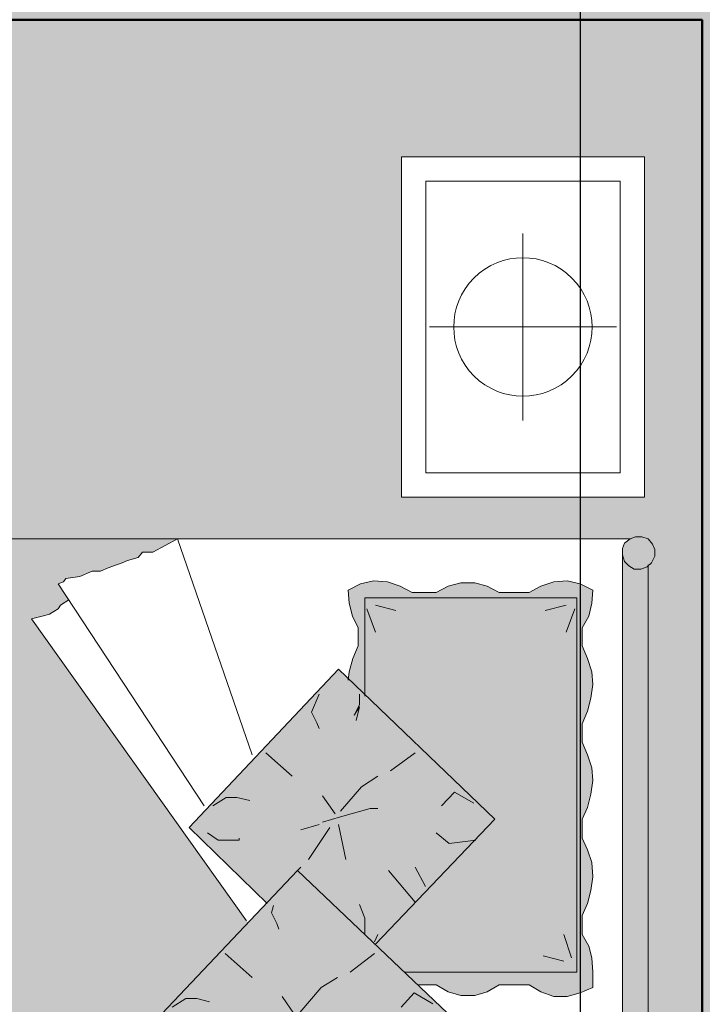
# Model space of a CAD drawing. Units: inches. Extents: x 528 to 2620, y -1066 to 798.
# Tile 30 of 41: x 1180 to 1211, y 665 to 710. Entities that reach past the tile are written whole.
import ezdxf

# ---------------------------------------------------------------- set-up
doc = ezdxf.new("R2010")
doc.units = ezdxf.units.IN
doc.header["$MEASUREMENT"] = 0
for name, color, linetype, lineweight in [('A-ANNO-DIMS', 2, 'Continuous', 18), ('A-FURN', 30, 'Continuous', 18), ('A-WALL', 7, 'Continuous', 50), ('A-WALL-PATT', 8, 'Continuous', 13)]:
    doc.layers.add(name, color=color, linetype=linetype, lineweight=lineweight)
doc.styles.get("Standard").update_dxf_attribs({"font": 'arial.ttf'})
doc.dimstyles.get("Standard").update_dxf_attribs({"dimtxt": 6, "dimasz": 2, "dimexe": 0.18, "dimexo": 0.0625, "dimgap": 0.09, "dimtad": 0, "dimtih": 1, "dimtoh": 1, "dimdec": 1, "dimzin": 0, "dimdsep": 46, "dimlunit": 3, "dimtxsty": 'Standard', "dimblk": 'ARCHTICK', "dimcen": 0.09, "dimadec": 0, "dimazin": 0, "dimtfac": 1, "dimtdec": 1, "dimtofl": 0, "dimtmove": 0, "dimatfit": 3, "dimfxl": 1, "dimtolj": 1, "dimtzin": 0, "dimarcsym": 0})

# ---------------------------------------------------------------- blocks, each defined once
blk = doc.blocks.new('d-bed-3')
at = {"color": 0, "linetype": 'ByBlock'}
for p, q in [((0.7968, 0.0166), (0.8078, 0.0211)), ((0.7968, 0.0166), (0.8078, 0.0211)), ((0.8078, 0.0211), (0.8209, 0.0211)), ((0.8078, 0.0211), (0.8209, 0.0211)), ((0.8209, 0.0211), (0.8349, 0.0144)), ((0.8209, 0.0211), (0.8349, 0.0144)), ((0, 0), (0, -0.5)), ((0.7, 0), (0, 0)), ((0.7, -0.5), (0.7, 0)), ((0.7817, -0.0054), (0.7857, 0.0078)), ((0.7817, -0.0054), (0.7857, 0.0078)), ((0.7857, 0.0078), (0.7968, 0.0166)), ((0.7857, 0.0078), (0.7968, 0.0166)), ((0.8349, 0.0144), (0.8409, 0.0078)), ((0.8349, 0.0144), (0.8429, 0.0056)), ((0.8389, 0.0078), (2.7305, 0.0078)), ((0.8409, 0.0078), (2.7305, 0.0078)), ((0.8429, 0.0056), (0.848, -0.0077)), ((0.7817, -0.0187), (0.7817, -0.0054)), ((0.7817, -0.0187), (0.7817, -0.0054)), ((0.7857, -0.0297), (0.7817, -0.0187)), ((0.7857, -0.0297), (0.7817, -0.0187)), ((0.848, -0.0077), (0.848, -0.0209)), ((0.7857, -2.0939), (0.7857, -0.0297)), ((0.7948, -0.0408), (0.7857, -0.0297)), ((0.7857, -0.032), (0.7857, -2.0939)), ((0.8409, -0.032), (0.8319, -0.0408)), ((0.848, -0.0209), (0.8409, -0.032)), ((0.05, -0.05), (0.05, -0.45)), ((0.65, -0.05), (0.05, -0.05)), ((0.35, -0.0576), (0.35, -0.4424)), ((0.65, -0.45), (0.65, -0.05)), ((0.8058, -0.0452), (0.7948, -0.0408)), ((0.8188, -0.0452), (0.8058, -0.0452)), ((0.8319, -0.0408), (0.8188, -0.0452)), ((2.7525, -0.0452), (0.8188, -0.0452)), ((0.8781, -0.1325), (0.8911, -0.1059)), ((0.8911, -0.1059), (0.9182, -0.1082)), ((0.9182, -0.1082), (0.9443, -0.1148)), ((0.9443, -0.1148), (0.9684, -0.128)), ((1.0056, -0.128), (1.0317, -0.117)), ((1.0317, -0.117), (1.0588, -0.1082)), ((1.0588, -0.1082), (1.0849, -0.1059)), ((1.0849, -0.1059), (1.113, -0.1104)), ((1.113, -0.1104), (1.1401, -0.117)), ((1.1401, -0.117), (1.1662, -0.128)), ((1.2034, -0.128), (1.2295, -0.117)), ((1.2295, -0.117), (1.2566, -0.1082)), ((1.2566, -0.1082), (1.2827, -0.1059)), ((1.2827, -0.1059), (1.3108, -0.1104)), ((1.3108, -0.1104), (1.3379, -0.117)), ((1.3379, -0.117), (1.362, -0.128)), ((1.4012, -0.128), (1.4253, -0.117)), ((1.4253, -0.117), (1.4514, -0.1082)), ((1.4514, -0.1082), (1.4805, -0.1059)), ((1.4805, -0.1059), (1.5086, -0.1104)), ((1.5086, -0.1104), (1.5357, -0.117)), ((1.5357, -0.117), (1.5598, -0.128)), ((1.5989, -0.128), (1.623, -0.1148)), ((1.623, -0.1148), (1.6471, -0.1082)), ((1.6471, -0.1082), (1.6763, -0.1059)), ((1.6763, -0.1059), (1.7084, -0.1059)), ((1.7084, -0.1059), (1.7194, -0.1325)), ((0.8721, -0.159), (0.8781, -0.1325)), ((0.9072, -0.5753), (0.9072, -0.1391)), ((0.9072, -0.1391), (1.6763, -0.1391)), ((0.9684, -0.128), (1.0056, -0.128)), ((1.1662, -0.128), (1.2034, -0.128)), ((1.362, -0.128), (1.4012, -0.128)), ((1.5598, -0.128), (1.5989, -0.128)), ((1.6763, -0.1391), (1.6763, -0.4936)), ((1.7194, -0.1325), (1.7265, -0.159)), ((0.8741, -0.1866), (0.8721, -0.159)), ((0.9223, -0.1612), (0.9333, -0.2042)), ((0.9293, -0.1435), (0.9775, -0.1612)), ((1.6471, -0.1501), (1.5989, -0.1656)), ((1.7265, -0.159), (1.7265, -0.1866)), ((1.6542, -0.1656), (1.6431, -0.2087)), ((0.8831, -0.2131), (0.8741, -0.1866)), ((1.7265, -0.1866), (1.7174, -0.2131)), ((0.8962, -0.2374), (0.8831, -0.2131)), ((1.7174, -0.2131), (1.7024, -0.2374)), ((0.8962, -0.2992), (0.8962, -0.2374)), ((1.7024, -0.2374), (1.7024, -0.2992)), ((0.1576, -0.25), (0.5424, -0.25)), ((0.8831, -0.3235), (0.8962, -0.2992)), ((1.7024, -0.2992), (1.7174, -0.3235)), ((0.8761, -0.3489), (0.8831, -0.3235)), ((1.0538, -0.6294), (1.362, -0.3081)), ((1.362, -0.3081), (1.619, -0.5532)), ((1.7174, -0.3235), (1.7244, -0.3489)), ((0.8761, -0.3776), (0.8761, -0.3489)), ((1.3289, -0.3511), (1.3068, -0.3909)), ((1.4052, -0.3467), (1.4122, -0.4019)), ((1.7244, -0.3489), (1.7244, -0.3776)), ((0.8831, -0.4041), (0.8761, -0.3776)), ((1.7244, -0.3776), (1.7174, -0.4041)), ((0.8962, -0.4284), (0.8831, -0.4041)), ((1.3068, -0.3909), (1.3349, -0.4174)), ((1.4122, -0.4019), (1.3901, -0.4284)), ((1.4674, -0.7134), (1.7746, -0.3909)), ((1.7174, -0.4041), (1.7024, -0.4284)), ((0.8962, -0.4781), (0.8962, -0.4284)), ((1.7024, -0.4284), (1.7024, -0.4649)), ((1.7415, -0.4351), (1.7194, -0.4737)), ((0.05, -0.45), (0.65, -0.45)), ((1.5006, -0.4505), (1.4604, -0.4715)), ((0.8831, -0.5024), (0.8962, -0.4781)), ((1.2255, -0.4715), (1.2626, -0.5223)), ((1.5327, -0.4715), (1.4674, -0.5267)), ((1.7194, -0.4737), (1.7485, -0.5002)), ((0, -0.5), (0.7, -0.5)), ((0.8741, -0.5289), (0.8831, -0.5024)), ((0.9223, -0.5532), (0.9333, -0.5113)), ((0.8721, -0.5576), (0.8741, -0.5289)), ((0.8781, -0.5841), (0.8721, -0.5576)), ((0.9293, -0.5709), (0.9775, -0.5532)), ((1.2957, -0.5819), (1.2737, -0.5488)), ((1.3399, -0.5643), (1.3399, -0.5488)), ((1.357, -0.625), (1.3399, -0.5643)), ((1.5989, -0.5488), (1.614, -0.5554)), ((1.6381, -0.5554), (1.6763, -0.6051)), ((0.8911, -0.6096), (0.8781, -0.5841)), ((1.109, -0.5753), (0.9072, -0.5753)), ((1.105, -0.5864), (1.1271, -0.5864)), ((1.1271, -0.5864), (1.1482, -0.5974)), ((1.1482, -0.5974), (1.1311, -0.5864)), ((1.1311, -0.5864), (1.1592, -0.593)), ((1.3459, -0.625), (1.2957, -0.5819)), ((1.5658, -0.5753), (1.5377, -0.5864)), ((1.5969, -0.5753), (1.5658, -0.5753)), ((0.9182, -0.6073), (0.8911, -0.6096)), ((0.9443, -0.6007), (0.9182, -0.6073)), ((0.9684, -0.5886), (0.9443, -0.6007)), ((1.0056, -0.5886), (0.9684, -0.5886)), ((1.0317, -0.5996), (1.0056, -0.5886)), ((1.0588, -0.6073), (1.0317, -0.5996)), ((1.0759, -0.6096), (1.0588, -0.6073)), ((1.368, -0.6626), (1.357, -0.625)), ((1.3731, -0.6294), (1.4453, -0.614)), ((1.3791, -0.9365), (1.0538, -0.6294)), ((1.3138, -0.6626), (1.351, -0.6361)), ((1.3791, -0.6471), (1.4453, -0.6913)), ((1.7084, -0.6648), (1.6873, -0.6316)), ((1.7596, -0.7089), (1.7084, -0.6648)), ((1.105, -0.6692), (1.1421, -0.6846)), ((1.1421, -0.6846), (1.1642, -0.6736)), ((1.1642, -0.6736), (1.1753, -0.6692)), ((1.3731, -0.6692), (1.3841, -0.7067)), ((1.4674, -0.7134), (1.4604, -0.7067)), ((1.2255, -0.7785), (1.2737, -0.7244)), ((1.7897, -1.0193), (1.4674, -0.7134)), ((1.7265, -0.7454), (1.7636, -0.72)), ((1.5548, -0.7675), (1.5397, -0.7631)), ((1.5548, -0.7675), (1.5769, -0.7564)), ((1.5769, -0.7564), (1.5879, -0.752)), ((1.3791, -0.9365), (1.5357, -0.7763)), ((0.7857, -0.9607), (1.2295, -0.8072)), ((1.6381, -0.8625), (1.6873, -0.8072)), ((0.9504, -1.2611), (1.5708, -0.8183)), ((1.3178, -0.8382), (1.3239, -0.8117)), ((1.3178, -0.8602), (1.3178, -0.8382)), ((1.4052, -0.8337), (1.4012, -0.8337)), ((1.4052, -0.8768), (1.4052, -0.8337)), ((1.3349, -0.8879), (1.3178, -0.8602)), ((1.3901, -0.8989), (1.4052, -0.8768)), ((0.8781, -1.2059), (1.3349, -0.9055)), ((1.7305, -0.921), (1.7375, -0.8945)), ((1.7305, -0.9431), (1.7305, -0.921)), ((1.7485, -0.9718), (1.7305, -0.9431)), ((0.8128, -1.0115), (0.7857, -0.9607)), ((0.8128, -1.0325), (0.8128, -1.0115)), ((0.8239, -1.0414), (0.8128, -1.0325)), ((0.8299, -1.0635), (0.8239, -1.0414)), ((0.8349, -1.0745), (0.8299, -1.0635)), ((0.845, -1.1032), (0.8349, -1.0745)), ((0.852, -1.1187), (0.845, -1.1032)), ((0.852, -1.1363), (0.852, -1.1187)), ((0.863, -1.1617), (0.852, -1.1363)), ((0.867, -1.1905), (0.863, -1.1617)), ((0.8741, -1.1949), (0.867, -1.1905)), ((0.9223, -1.2015), (0.9112, -1.1838)), ((0.8781, -1.2059), (0.8741, -1.1949)), ((0.9293, -1.2059), (0.9223, -1.2015)), ((0.9403, -1.2236), (0.9293, -1.2059)), ((0.9443, -1.2391), (0.9403, -1.2236)), ((0.9504, -1.2611), (0.9443, -1.2391))]:
    blk.add_line(p, q, dxfattribs=at)
blk.add_ellipse((0.35, -0.25), major_axis=(-0.1007, 0.1007), ratio=1, dxfattribs=at)
blk = doc.blocks.new('_ArchTick')
at = {"color": 0, "linetype": 'ByBlock', "const_width": 0.15}
blk.add_lwpolyline([(-0.5, -0.5), (0.5, 0.5)], dxfattribs=at)
blk = doc.blocks.new('*D42')
at = {"layer": 'A-ANNO-DIMS', "color": 0, "lineweight": -2, "transparency": 16777216}
for p, q in [((1159.521, 703.64), (1147.464, 703.64)), ((1147.644, 703.64), (1147.644, 667.032)), ((1147.644, 624.039), (1147.644, 660.647)), ((1159.521, 624.039), (1147.464, 624.039))]:
    blk.add_line(p, q, dxfattribs=at)
at = {"layer": 'Defpoints', "color": 0, "transparency": 16777216}
for p in [(1159.584, 703.64), (1147.644, 624.039), (1159.584, 624.039)]:
    blk.add_point(p, dxfattribs=at)
at = {"layer": 'A-ANNO-DIMS', "color": 0, "lineweight": -2, "transparency": 16777216, "xscale": 2, "yscale": 2, "zscale": 2}
for p, rotation in [((1147.644, 703.64), 90), ((1147.644, 624.039), 270)]:
    blk.add_blockref('_ArchTick', p, dxfattribs=dict(at, rotation=rotation))
at = {"layer": 'A-ANNO-DIMS', "color": 0, "transparency": 16777216, "insert": (1147.644, 663.839), "char_height": 6, "attachment_point": 5}
blk.add_mtext('\\A1;BED 6\'-7 1/2" TYP.', dxfattribs=at)
blk = doc.blocks.new('*D58')
at = {"layer": 'A-ANNO-DIMS', "color": 0, "lineweight": -2, "transparency": 16777216}
for p, q in [((1165.496, 577.985), (1165.496, 751.102)), ((1165.496, 750.922), (1177.395, 750.922)), ((1205.418, 750.922), (1193.52, 750.922)), ((1205.418, 577.985), (1205.418, 751.102))]:
    blk.add_line(p, q, dxfattribs=at)
at = {"layer": 'Defpoints', "color": 0, "transparency": 16777216}
for p in [(1205.418, 750.922), (1165.496, 577.922), (1205.418, 577.922)]:
    blk.add_point(p, dxfattribs=at)
at = {"layer": 'A-ANNO-DIMS', "color": 0, "lineweight": -2, "transparency": 16777216, "xscale": 2, "yscale": 2, "zscale": 2, "rotation": 180}
blk.add_blockref('_ArchTick', (1165.496, 750.922), dxfattribs=at)
at = {"layer": 'A-ANNO-DIMS', "color": 0, "lineweight": -2, "transparency": 16777216, "xscale": 2, "yscale": 2, "zscale": 2}
blk.add_blockref('_ArchTick', (1205.418, 750.922), dxfattribs=at)
at = {"layer": 'A-ANNO-DIMS', "color": 0, "transparency": 16777216, "insert": (1185.457, 750.922), "char_height": 6, "attachment_point": 5}
blk.add_mtext('\\A1;3\'-4"', dxfattribs=at)

msp = doc.modelspace()

# ---------------------------------------------------------------- hatches: boundary and pattern name
at = {"layer": 'A-WALL-PATT', "transparency": 33554521}
h = msp.add_hatch(color=256, dxfattribs=at)
h.dxf.hatch_style = 1
h.paths.add_polyline_path([(1065.996, 709.922), (1114.496, 709.922), (1114.496, 718.922), (1056.996, 718.922), (1056.996, 667.922), (1065.996, 667.922)])
h.paths.add_polyline_path([(1227.496, 718.922), (1162.496, 718.922), (1162.496, 709.922), (1210.996, 709.922), (1210.996, 577.922), (1205.418, 577.922), (1205.496, 573.422), (1210.996, 573.422), (1210.996, 567.422), (1215.496, 567.422), (1215.496, 669.422), (1267.996, 669.422), (1267.996, 675.922), (1263.496, 675.922), (1263.496, 673.922), (1215.496, 673.922), (1215.496, 709.922), (1227.496, 709.922)])
h.paths.add_polyline_path([(1344.996, 718.922), (1315.996, 718.922), (1315.996, 709.922), (1335.996, 709.922), (1335.996, 641.672), (1344.996, 641.672)])
h.paths.add_polyline_path([(1065.996, 619.922), (1056.996, 619.922), (1056.996, 561.422), (1065.996, 561.422), (1065.996, 573.422), (1160.996, 573.422), (1160.996, 569.422), (1165.496, 569.422), (1165.496, 577.922), (1065.996, 577.922)])
h.paths.add_polyline_path([(1215.996, 391.422), (1215.996, 400.422), (1206.996, 400.422), (1200.996, 400.422), (1200.996, 397.422), (1200.996, 391.422), (1206.996, 391.422), (1206.996, 268.922), (1251.996, 268.922), (1251.996, 277.922), (1215.996, 277.922), (1215.996, 359.767)])
h.paths.add_polyline_path([(1344.996, 395.922), (1335.996, 395.922), (1287.996, 395.922), (1287.996, 391.422), (1335.996, 391.422), (1335.996, 277.922), (1299.996, 277.922), (1299.996, 268.922), (1344.996, 268.922)])
h.paths.add_polyline_path([(1344.996, 593.672), (1335.996, 593.672), (1335.996, 525.422), (1215.496, 525.422), (1215.496, 527.172), (1210.996, 527.172), (1210.996, 520.922), (1335.996, 520.922), (1335.996, 443.922), (1344.996, 443.922)])
h.paths.add_polyline_path([(1065.996, 520.922), (1165.496, 520.922), (1165.496, 545.422), (1160.996, 545.422), (1160.996, 525.422), (1065.996, 525.422), (1065.996, 537.422), (1056.996, 537.422), (1056.996, 484.672), (1065.996, 484.672)])
h.paths.add_polyline_path([(1065.996, 436.672), (1056.996, 436.672), (1056.996, 391.422), (1085.496, 391.422), (1085.496, 400.422), (1065.996, 400.422)])
h.paths.add_polyline_path([(1152.996, 397.422), (1152.996, 400.422), (1133.496, 400.422), (1133.496, 391.422), (1152.996, 391.422)])
at = {"layer": 'A-WALL-PATT', "transparency": 33554536}
h = msp.add_hatch(color=256, dxfattribs=at)
h.dxf.hatch_style = 1
h.paths.add_polyline_path([(1335.996, 709.922), (1267.996, 709.922), (1267.996, 699.922), (1266.746, 699.922), (1266.746, 675.922), (1267.996, 675.922), (1267.996, 669.422), (1215.496, 669.422), (1215.496, 567.172), (1216.996, 567.172), (1256.996, 567.172), (1256.996, 565.422), (1256.958, 565.422, -0.401453), (1216.996, 527.172), (1215.496, 527.172), (1215.496, 525.422), (1335.996, 525.422)], flags=17)
h.paths.add_polyline_path([(1285.032, 635.927), (1285.229, 636.128), (1285.672, 636.263), (1286.206, 636.02), (1286.976, 636.084), (1332.983, 636.084), (1333.363, 636.222), (1333.82, 636.084), (1334.115, 635.714), (1334.115, 635.3), (1333.907, 634.86), (1333.82, 634.827), (1333.82, 592.738), (1333.967, 592.604), (1334.115, 592.291), (1334.115, 591.877), (1333.82, 591.507), (1333.363, 591.369), (1332.983, 591.507), (1332.638, 591.789), (1332.638, 591.507), (1286.976, 591.507), (1286.173, 591.672), (1286.066, 591.574), (1285.681, 591.37), (1285.229, 591.507), (1285.032, 591.709), (1284.834, 592.098), (1284.983, 592.537), (1285.13, 592.688), (1285.13, 634.948), (1284.983, 635.099), (1284.834, 635.537)], flags=16)
h.paths.add_polyline_path([(1285.032, 635.927), (1285.229, 636.128), (1285.672, 636.263), (1286.206, 636.02), (1286.976, 636.084), (1332.983, 636.084), (1333.363, 636.222), (1333.82, 636.084), (1334.115, 635.714), (1334.115, 635.3), (1333.967, 634.987), (1333.82, 634.853), (1333.82, 592.738), (1333.967, 592.604), (1334.115, 592.291), (1334.115, 591.877), (1333.82, 591.507), (1333.363, 591.369), (1332.983, 591.507), (1332.638, 591.789), (1332.638, 592.246), (1332.638, 635.345), (1332.638, 635.802), (1332.983, 636.084), (1312.232, 636.084), (1311.1, 635.479), (1310.632, 635.479), (1310.435, 635.233), (1309.943, 635.099), (1309.696, 634.987), (1309.056, 634.763), (1308.712, 634.607), (1308.318, 634.607), (1307.752, 634.36), (1307.112, 634.271), (1307.013, 634.114), (1306.767, 634.025), (1307.255, 633.283), (1306.866, 633.04), (1306.767, 632.884), (1306.373, 632.637), (1306.029, 632.548), (1305.536, 632.414), (1315.472, 618.494), (1316.321, 619.388), (1312.773, 622.858), (1319.616, 630.109), (1320.067, 629.676), (1320.109, 629.997), (1320.281, 630.601), (1320.527, 631.183), (1320.527, 632.011), (1320.256, 632.548), (1320.109, 633.13), (1320.06, 633.734), (1320.626, 634.025), (1321.216, 634.159), (1321.856, 634.114), (1322.447, 633.913), (1322.989, 633.622), (1324.096, 633.622), (1324.638, 633.913), (1325.229, 634.07), (1325.869, 634.07), (1326.435, 633.913), (1326.976, 633.622), (1328.355, 633.622), (1328.896, 633.913), (1329.487, 634.114), (1330.103, 634.159), (1330.693, 634.025), (1331.284, 633.734), (1331.235, 633.13), (1331.087, 632.548), (1330.792, 632.011), (1330.792, 631.183), (1331.038, 630.601), (1331.235, 629.997), (1331.284, 629.415), (1331.186, 628.788), (1331.038, 628.184), (1330.792, 627.602), (1330.792, 626.774), (1331.038, 626.193), (1331.235, 625.588), (1331.284, 625.007), (1331.186, 624.38), (1331.038, 623.776), (1330.792, 623.239), (1330.792, 622.366), (1331.038, 621.829), (1331.235, 621.247), (1331.284, 620.598), (1331.186, 619.972), (1331.038, 619.367), (1330.792, 618.83), (1330.792, 617.958), (1331.087, 617.421), (1331.235, 616.884), (1331.284, 616.235), (1331.284, 615.518), (1330.693, 615.272), (1330.103, 615.116), (1329.487, 615.116), (1328.896, 615.317), (1328.355, 615.653), (1326.976, 615.653), (1326.435, 615.317), (1325.869, 615.16), (1325.229, 615.16), (1324.638, 615.317), (1324.096, 615.653), (1323.242, 615.653), (1324.933, 614.042), (1322.978, 611.983), (1324.096, 611.983), (1324.638, 612.274), (1325.278, 612.43), (1325.869, 612.43), (1326.484, 612.274), (1327.026, 611.983), (1328.355, 611.983), (1328.896, 612.274), (1329.487, 612.475), (1330.103, 612.52), (1330.743, 612.386), (1331.284, 612.072), (1331.284, 611.356), (1331.284, 610.752), (1331.087, 610.17), (1330.792, 609.633), (1330.792, 608.805), (1331.087, 608.223), (1331.235, 607.619), (1331.284, 606.993), (1331.235, 606.411), (1331.087, 605.807), (1330.792, 605.225), (1330.792, 604.397), (1331.087, 603.815), (1331.235, 603.211), (1331.284, 602.629), (1331.235, 602.002), (1331.087, 601.398), (1330.792, 600.861), (1330.792, 599.988), (1331.087, 599.451), (1331.235, 598.87), (1331.284, 598.221), (1331.235, 597.594), (1331.087, 596.99), (1330.792, 596.453), (1330.792, 595.58), (1331.087, 595.043), (1331.284, 594.506), (1331.284, 593.857), (1330.743, 593.611), (1330.103, 593.477), (1329.487, 593.477), (1328.896, 593.678), (1328.355, 594.014), (1327.026, 594.014), (1326.484, 593.678), (1325.869, 593.521), (1325.278, 593.521), (1324.638, 593.678), (1324.096, 594.014), (1323.038, 594.014), (1322.496, 593.678), (1321.906, 593.477), (1321.266, 593.477), (1320.626, 593.611), (1320.109, 593.857), (1320.109, 594.506), (1320.281, 595.043), (1320.576, 595.58), (1320.576, 596.453), (1320.281, 596.99), (1320.158, 597.594), (1320.104, 598.015), (1319.616, 597.549), (1315.659, 601.729), (1312.232, 591.574), (1311.74, 591.664), (1311.592, 591.91), (1310.78, 592.402), (1309.549, 592.895), (1308.958, 592.895), (1308.712, 593.029), (1308.564, 593.141), (1307.752, 593.521), (1306.767, 593.611), (1307.248, 594.356), (1306.866, 594.595), (1306.373, 594.842), (1306.029, 595.088), (1305.536, 595.244), (1315.465, 609.354), (1310.927, 613.706), (1315.472, 618.494), (1305.536, 632.414), (1306.029, 632.548), (1306.373, 632.637), (1306.767, 632.884), (1306.866, 633.04), (1307.255, 633.283), (1306.767, 634.025), (1307.013, 634.114), (1307.112, 634.271), (1307.752, 634.36), (1308.318, 634.607), (1308.712, 634.607), (1309.056, 634.763), (1309.696, 634.987), (1309.943, 635.099), (1310.435, 635.233), (1310.632, 635.479), (1311.1, 635.479), (1312.232, 636.084), (1286.976, 636.084), (1286.216, 636.021), (1286.411, 635.444), (1286.213, 635.054), (1286.016, 634.853), (1285.869, 634.808), (1285.869, 592.839), (1286.153, 592.731), (1286.41, 592.188), (1286.231, 591.66), (1286.173, 591.672), (1286.066, 591.574), (1285.681, 591.37), (1285.229, 591.507), (1285.032, 591.709), (1284.834, 592.098), (1284.983, 592.537), (1285.13, 592.688), (1285.13, 634.948), (1284.983, 635.099), (1284.834, 635.537)], flags=0)
h.paths.add_polyline_path([(1322.501, 653.596), (1333.646, 653.596), (1333.646, 637.994), (1322.501, 637.994)], flags=16)
h.paths.add_polyline_path([(1323.616, 652.482), (1332.531, 652.482), (1332.531, 639.108), (1323.616, 639.108)], flags=0)
edge = h.paths.add_edge_path(flags=0)
edge.add_ellipse((1328.073, 645.795), major_axis=(2.245, 2.245), ratio=1, start_angle=405, end_angle=495, ccw=False)
edge.add_ellipse((1328.073, 645.795), major_axis=(2.245, 2.245), ratio=1, start_angle=675, end_angle=765, ccw=False)
edge.add_ellipse((1328.073, 645.795), major_axis=(2.245, 2.245), ratio=1, start_angle=585, end_angle=675, ccw=False)
edge.add_ellipse((1328.073, 645.795), major_axis=(2.245, 2.245), ratio=1, start_angle=495, end_angle=585, ccw=False)
h.paths.add_polyline_path([(1320.576, 628.386), (1320.33, 628.005), (1320.615, 628.548)], flags=0)
h.paths.add_polyline_path([(1317.893, 604.889), (1318.78, 604.643), (1319.764, 604.285), (1318.878, 604.531)], flags=0)
h.paths.add_polyline_path([(1320.33, 599.653), (1320.576, 599.25), (1320.576, 599.16)], flags=0)
h.paths.add_polyline_path([(1322.501, 589.597), (1333.646, 589.597), (1333.646, 573.995), (1322.501, 573.995)], flags=16)
h.paths.add_polyline_path([(1323.616, 588.482), (1332.531, 588.482), (1332.531, 575.109), (1323.616, 575.109)], flags=0)
edge = h.paths.add_edge_path(flags=0)
edge.add_ellipse((1328.073, 581.796), major_axis=(-2.245, 2.245), ratio=1, start_angle=-45, end_angle=45, ccw=False)
edge.add_ellipse((1328.073, 581.796), major_axis=(-2.245, 2.245), ratio=1, start_angle=-135, end_angle=-45, ccw=False)
edge.add_ellipse((1328.073, 581.796), major_axis=(-2.245, 2.245), ratio=1, start_angle=135, end_angle=-135, ccw=False)
edge.add_ellipse((1328.073, 581.796), major_axis=(-2.245, 2.245), ratio=1, start_angle=45, end_angle=135, ccw=False)
h.paths.add_polyline_path([(1264.746, 699.922), (1263.496, 699.922), (1263.496, 709.922), (1215.496, 709.922), (1215.496, 673.922), (1263.496, 673.922), (1263.496, 675.922), (1264.746, 675.922)], flags=16)
h.paths.add_polyline_path([(1162.192, 569.422), (1160.996, 569.422), (1160.996, 573.422), (1065.996, 573.422), (1065.996, 525.422), (1160.996, 525.422), (1160.996, 545.422), (1162.192, 545.422)])
h.paths.add_polyline_path([(1256.958, 565.422), (1256.996, 565.422), (1256.996, 567.172), (1216.996, 567.172), (1215.496, 567.172), (1215.496, 567.422), (1210.996, 567.422), (1210.996, 573.422), (1205.496, 573.422), (1205.418, 577.922), (1210.996, 577.922), (1210.996, 709.922), (1065.996, 709.922), (1065.996, 577.922), (1165.496, 577.922), (1165.496, 569.422), (1164.192, 569.422), (1164.192, 545.422), (1165.496, 545.422), (1165.496, 520.922), (1152.996, 520.922), (1152.996, 484.922), (1101.996, 484.922), (1101.996, 436.422), (1152.996, 436.422), (1152.996, 400.422), (1152.996, 391.422), (1200.996, 391.422), (1200.996, 400.422), (1206.996, 400.422), (1215.996, 400.422), (1215.996, 391.422), (1215.996, 277.922), (1335.996, 277.922), (1335.996, 391.422), (1287.996, 391.422), (1287.996, 395.922), (1335.996, 395.922), (1335.996, 443.922), (1335.996, 520.922), (1210.996, 520.922), (1210.996, 527.172), (1215.496, 527.172), (1216.996, 527.172, 0.401453)])
h.paths.add_polyline_path([(1167.246, 579.422), (1165.496, 579.422), (1165.496, 619.422), (1167.246, 619.422)], flags=16)
h.paths.add_polyline_path([(1227.97, 501.564), (1236.36, 502.031), (1236.36, 492.555), (1227.97, 493.021, -0.254069)], flags=16)
h.paths.add_polyline_path([(1243.336, 515.692, -0.254069), (1251.879, 515.692), (1252.345, 507.301), (1242.87, 507.301)], flags=16)
h.paths.add_polyline_path([(1239.185, 504.685), (1256.03, 504.685), (1256.03, 479.416), (1239.185, 479.416)], flags=16)
h.paths.add_polyline_path([(1227.97, 489.602), (1236.36, 490.068), (1236.36, 480.592), (1227.97, 481.058, -0.254069)], flags=16)
h.paths.add_polyline_path([(1197.201, 624.039), (1197.201, 639.641), (1208.345, 639.641), (1208.345, 624.039)], flags=16)
h.paths.add_polyline_path([(1198.315, 625.153), (1198.315, 638.526), (1207.231, 638.526), (1207.231, 625.153)], flags=0)
h.paths.add_polyline_path([(1258.855, 502.031), (1267.245, 501.564, -0.254069), (1267.245, 493.021), (1258.855, 492.555)], flags=16)
h.paths.add_polyline_path([(1271.589, 519.657), (1333.671, 519.657), (1333.671, 451.595), (1319.087, 451.595), (1319.087, 505.072), (1288.093, 505.072), (1284.447, 505.072, -0.883215), (1270.678, 514.188), (1270.678, 518.745, -0.414214)], flags=16)
h.paths.add_polyline_path([(1331.848, 517.834), (1331.848, 453.418), (1328.202, 453.418), (1328.202, 505.072), (1298.424, 505.072), (1298.424, 514.188), (1288.093, 514.188), (1288.093, 517.834)], flags=0)
h.paths.add_polyline_path([(1242.87, 476.8), (1252.345, 476.8), (1251.879, 468.409, -0.254069), (1243.336, 468.409)], flags=16)
h.paths.add_polyline_path([(1258.855, 490.068), (1267.245, 489.602, -0.254069), (1267.245, 481.058), (1258.855, 480.592)], flags=16)
h.paths.add_polyline_path([(1161.676, 641.551), (1160.873, 641.716), (1160.765, 641.618), (1160.38, 641.414), (1159.928, 641.551), (1159.731, 641.753), (1159.534, 642.142), (1159.682, 642.581), (1159.83, 642.732), (1159.83, 684.992), (1159.682, 685.143), (1159.534, 685.582), (1159.731, 685.971), (1159.928, 686.172), (1160.371, 686.307), (1160.905, 686.064), (1161.676, 686.128), (1207.682, 686.128), (1208.063, 686.266), (1208.519, 686.128), (1208.815, 685.758), (1208.815, 685.344), (1208.607, 684.904), (1208.519, 684.871), (1208.519, 642.782), (1208.667, 642.648), (1208.877, 642.201), (1208.716, 641.797), (1208.519, 641.551), (1208.063, 641.413), (1207.682, 641.551), (1207.338, 641.833), (1207.338, 641.551)], flags=16)
h.paths.add_polyline_path([(1186.931, 641.618), (1186.439, 641.708), (1186.291, 641.954), (1185.479, 642.446), (1184.248, 642.939), (1183.658, 642.939), (1183.411, 643.073), (1183.264, 643.185), (1182.451, 643.565), (1181.467, 643.655), (1181.948, 644.4), (1181.565, 644.639), (1181.073, 644.886), (1180.728, 645.132), (1180.236, 645.288), (1190.164, 659.398), (1185.627, 663.75), (1190.171, 668.538), (1180.236, 682.458), (1180.728, 682.592), (1181.073, 682.681), (1181.467, 682.928), (1181.565, 683.084), (1181.954, 683.327), (1181.467, 684.069), (1181.713, 684.158), (1181.811, 684.315), (1182.451, 684.404), (1183.018, 684.651), (1183.411, 684.651), (1183.756, 684.807), (1184.396, 685.031), (1184.642, 685.143), (1185.135, 685.277), (1185.331, 685.523), (1185.799, 685.523), (1186.931, 686.128), (1161.676, 686.128), (1160.915, 686.065), (1161.111, 685.488), (1160.913, 685.098), (1160.716, 684.897), (1160.568, 684.852), (1160.568, 642.883), (1160.853, 642.775), (1161.109, 642.232), (1160.931, 641.704), (1160.873, 641.716), (1160.765, 641.618), (1160.38, 641.414), (1159.928, 641.551), (1159.731, 641.753), (1159.534, 642.142), (1159.682, 642.581), (1159.83, 642.732), (1159.83, 684.992), (1159.682, 685.143), (1159.534, 685.582), (1159.731, 685.971), (1159.928, 686.172), (1160.371, 686.307), (1160.905, 686.064), (1161.676, 686.128), (1207.682, 686.128), (1208.063, 686.266), (1208.519, 686.128), (1208.815, 685.758), (1208.815, 685.344), (1208.667, 685.031), (1208.519, 684.897), (1208.519, 642.782), (1208.667, 642.648), (1208.877, 642.201), (1208.716, 641.797), (1208.519, 641.551), (1208.063, 641.413), (1207.682, 641.551), (1207.338, 641.833), (1207.338, 642.29), (1207.338, 685.389), (1207.338, 685.846), (1207.682, 686.128), (1186.931, 686.128), (1185.799, 685.523), (1185.331, 685.523), (1185.135, 685.277), (1184.642, 685.143), (1184.396, 685.031), (1183.756, 684.807), (1183.411, 684.651), (1183.018, 684.651), (1182.451, 684.404), (1181.811, 684.315), (1181.713, 684.158), (1181.467, 684.069), (1181.954, 683.327), (1181.565, 683.084), (1181.467, 682.928), (1181.073, 682.681), (1180.728, 682.592), (1180.236, 682.458), (1190.171, 668.538), (1191.021, 669.432), (1187.473, 672.902), (1194.316, 680.153), (1194.767, 679.72), (1194.808, 680.041), (1194.981, 680.645), (1195.227, 681.227), (1195.227, 682.055), (1194.956, 682.592), (1194.808, 683.174), (1194.759, 683.778), (1195.325, 684.069), (1195.916, 684.203), (1196.556, 684.158), (1197.147, 683.957), (1197.688, 683.666), (1198.796, 683.666), (1199.338, 683.957), (1199.928, 684.114), (1200.568, 684.114), (1201.135, 683.957), (1201.676, 683.666), (1203.055, 683.666), (1203.596, 683.957), (1204.187, 684.158), (1204.802, 684.203), (1205.393, 684.069), (1205.984, 683.778), (1205.935, 683.174), (1205.787, 682.592), (1205.491, 682.055), (1205.491, 681.227), (1205.738, 680.645), (1205.935, 680.041), (1205.984, 679.459), (1205.885, 678.832), (1205.738, 678.228), (1205.491, 677.646), (1205.491, 676.818), (1205.738, 676.237), (1205.935, 675.632), (1205.984, 675.051), (1205.885, 674.424), (1205.738, 673.82), (1205.491, 673.283), (1205.491, 672.41), (1205.738, 671.873), (1205.935, 671.291), (1205.984, 670.642), (1205.885, 670.016), (1205.738, 669.411), (1205.491, 668.874), (1205.491, 668.002), (1205.787, 667.465), (1205.935, 666.928), (1205.984, 666.279), (1205.984, 665.563), (1205.393, 665.316), (1204.802, 665.16), (1204.187, 665.16), (1203.596, 665.361), (1203.055, 665.697), (1201.676, 665.697), (1201.135, 665.361), (1200.568, 665.204), (1199.928, 665.204), (1199.338, 665.361), (1198.796, 665.697), (1197.942, 665.697), (1199.633, 664.086), (1197.678, 662.027), (1198.796, 662.027), (1199.338, 662.318), (1199.978, 662.474), (1200.568, 662.474), (1201.184, 662.318), (1201.725, 662.027), (1203.055, 662.027), (1203.596, 662.318), (1204.187, 662.519), (1204.802, 662.564), (1205.442, 662.43), (1205.984, 662.116), (1205.984, 661.4), (1205.984, 660.796), (1205.787, 660.214), (1205.491, 659.677), (1205.491, 658.849), (1205.787, 658.267), (1205.935, 657.663), (1205.984, 657.037), (1205.935, 656.455), (1205.787, 655.851), (1205.491, 655.269), (1205.491, 654.441), (1205.787, 653.859), (1205.935, 653.255), (1205.984, 652.673), (1205.935, 652.046), (1205.787, 651.442), (1205.491, 650.905), (1205.491, 650.032), (1205.787, 649.495), (1205.935, 648.914), (1205.984, 648.265), (1205.935, 647.638), (1205.787, 647.034), (1205.491, 646.497), (1205.491, 645.624), (1205.787, 645.087), (1205.984, 644.55), (1205.984, 643.901), (1205.442, 643.655), (1204.802, 643.521), (1204.187, 643.521), (1203.596, 643.722), (1203.055, 644.058), (1201.725, 644.058), (1201.184, 643.722), (1200.568, 643.565), (1199.978, 643.565), (1199.338, 643.722), (1198.796, 644.058), (1197.738, 644.058), (1197.196, 643.722), (1196.605, 643.521), (1195.965, 643.521), (1195.325, 643.655), (1194.808, 643.901), (1194.808, 644.55), (1194.981, 645.087), (1195.276, 645.624), (1195.276, 646.497), (1194.981, 647.034), (1194.858, 647.638), (1194.803, 648.059), (1194.316, 647.593), (1190.359, 651.773)], flags=16)
h.paths.add_polyline_path([(1195.276, 649.204), (1195.03, 649.697), (1195.276, 649.294)], flags=0)
h.paths.add_polyline_path([(1194.464, 654.329), (1193.578, 654.575), (1192.593, 654.933), (1193.479, 654.687)], flags=0)
h.paths.add_polyline_path([(1195.276, 678.43), (1195.03, 678.049), (1195.314, 678.592)], flags=0)
h.paths.add_polyline_path([(1197.201, 688.038), (1197.201, 703.64), (1208.345, 703.64), (1208.345, 688.038)], flags=16)
h.paths.add_polyline_path([(1198.315, 689.152), (1198.315, 702.526), (1207.231, 702.526), (1207.231, 689.152)], flags=0)
h.paths.add_polyline_path([(1217.099, 329.02), (1230.651, 329.02), (1230.651, 315.468), (1217.099, 315.468)], flags=16)
h.paths.add_polyline_path([(1223.875, 322.244), (1227.263, 322.244), (1227.263, 321.322, -0.414214), (1229.729, 318.856, -1), (1224.797, 318.856), (1223.875, 318.856)], flags=0)
h.paths.add_polyline_path([(1222.115, 325.632, -1), (1218.859, 325.632, -1)], flags=0)
h.paths.add_polyline_path([(1228.25, 325.632, -1), (1226.276, 325.632, -1)], flags=0)
h.paths.add_polyline_path([(1221.533, 318.856, -1), (1219.441, 318.856, -1)], flags=0)
h.paths.add_polyline_path([(1299.145, 293.732), (1299.145, 278.539), (1271.232, 278.539), (1271.232, 293.732)], flags=16)
h.paths.add_polyline_path([(1259.687, 292.213), (1270.624, 292.213, -1), (1270.624, 291.605), (1259.687, 291.605, -1)], flags=16)
h.paths.add_polyline_path([(1259.687, 291.301), (1270.624, 291.301, -1), (1270.624, 290.693), (1259.687, 290.693, -1)], flags=16)
h.paths.add_polyline_path([(1259.687, 290.389), (1270.624, 290.389, -1), (1270.624, 289.782), (1259.687, 289.782, -1)], flags=16)
h.paths.add_polyline_path([(1259.687, 289.478), (1270.624, 289.478, -1), (1270.624, 288.87), (1259.687, 288.87, -1)], flags=16)
h.paths.add_polyline_path([(1259.687, 288.566), (1270.624, 288.566, -1), (1270.624, 287.958), (1259.687, 287.958, -1)], flags=16)
h.paths.add_polyline_path([(1274.406, 292.381), (1283.251, 292.381, -0.414214), (1285.074, 290.558), (1285.074, 283.642, -0.414214), (1283.251, 281.819), (1277.723, 281.819), (1278.673, 280.869, -0.57735), (1279.382, 280.16), (1279.436, 280.106, -1), (1279.027, 279.696), (1278.972, 279.751, -0.57735), (1278.263, 280.46), (1276.904, 281.819), (1274.406, 281.819, -0.414214), (1272.583, 283.642), (1272.583, 290.558, -0.414214)], flags=0)
h.paths.add_polyline_path([(1259.687, 287.655), (1270.624, 287.655, -1), (1270.624, 287.047), (1259.687, 287.047, -1)], flags=16)
h.paths.add_polyline_path([(1259.687, 286.743), (1270.624, 286.743, -1), (1270.624, 286.135), (1259.687, 286.135, -1)], flags=16)
h.paths.add_polyline_path([(1259.687, 285.831), (1270.624, 285.831, -1), (1270.624, 285.224), (1259.687, 285.224, -1)], flags=16)
h.paths.add_polyline_path([(1259.687, 284.92), (1270.624, 284.92, -1), (1270.624, 284.312), (1259.687, 284.312, -1)], flags=16)
h.paths.add_polyline_path([(1259.687, 284.008), (1270.624, 284.008, -1), (1270.624, 283.401), (1259.687, 283.401, -1)], flags=16)
h.paths.add_polyline_path([(1287.823, 292.381), (1296.669, 292.381, -0.414214), (1298.492, 290.558), (1298.492, 283.642, -0.414214), (1296.669, 281.819), (1291.14, 281.819), (1292.09, 280.869, -0.57735), (1292.799, 280.16), (1292.854, 280.106, -1), (1292.445, 279.696), (1292.39, 279.751, -0.57735), (1291.681, 280.46), (1290.322, 281.819), (1287.823, 281.819, -0.414214), (1286, 283.642), (1286, 290.558, -0.414214)], flags=0)
h.paths.add_polyline_path([(1259.687, 283.097), (1270.624, 283.097, -1), (1270.624, 282.489), (1259.687, 282.489, -1)], flags=16)
h.paths.add_polyline_path([(1279.939, 287.607, -1), (1278.01, 287.607, -1)], flags=0)
h.paths.add_polyline_path([(1259.687, 282.185), (1270.624, 282.185, -1), (1270.624, 281.577), (1259.687, 281.577, -1)], flags=16)
h.paths.add_polyline_path([(1259.687, 281.273), (1270.624, 281.273, -1), (1270.624, 280.666), (1259.687, 280.666, -1)], flags=16)
h.paths.add_polyline_path([(1275.156, 284.169, -1), (1274.77, 284.169, -1)], flags=0)
h.paths.add_polyline_path([(1293.357, 287.607, -1), (1291.427, 287.607, -1)], flags=0)
h.paths.add_polyline_path([(1275.144, 280.503), (1276.335, 280.503, -5.828427), (1276.335, 280.117), (1275.144, 280.117, -1)], flags=0)
h.paths.add_polyline_path([(1288.574, 284.169, -1), (1288.188, 284.169, -1)], flags=0)
h.paths.add_polyline_path([(1281.31, 280.503), (1282.501, 280.503, -1), (1282.501, 280.117), (1281.31, 280.117, -5.828427)], flags=0)
h.paths.add_polyline_path([(1288.562, 280.503), (1289.752, 280.503, -5.828427), (1289.752, 280.117), (1288.562, 280.117, -1)], flags=0)
h.paths.add_polyline_path([(1294.727, 280.503), (1295.918, 280.503, -1), (1295.918, 280.117), (1294.727, 280.117, -5.828427)], flags=0)
h.paths.add_polyline_path([(1206.996, 391.422), (1200.996, 391.422), (1061.496, 391.422), (1061.496, 307.96), (1068.996, 307.96), (1068.996, 305.422), (1206.996, 305.422)])
at = {"layer": 'A-WALL-PATT', "transparency": 33554480}
h = msp.add_hatch(color=256, dxfattribs=at)
h.dxf.hatch_style = 1
h.paths.add_polyline_path([(1210.996, 709.922), (1065.996, 709.922), (1065.996, 577.922), (1165.496, 577.922), (1165.496, 579.422), (1165.496, 619.422), (1167.246, 619.422), (1167.246, 619.384, -0.401453), (1205.496, 579.422), (1205.496, 577.922), (1210.996, 577.922)])
h.paths.add_polyline_path([(1160.833, 686.058), (1160.905, 686.064), (1160.765, 686.128)], flags=16)
h.paths.add_polyline_path([(1160.931, 641.704), (1160.931, 641.707), (1160.928, 641.705)], flags=0)
h.paths.add_polyline_path([(1159.83, 684.992), (1159.584, 685.244), (1159.584, 685.82), (1160.016, 686.262), (1160.224, 686.262), (1159.928, 686.172), (1159.731, 685.971), (1159.584, 685.68), (1159.584, 685.434), (1159.682, 685.143), (1159.879, 684.942), (1160.175, 684.807), (1160.421, 684.807), (1160.716, 684.897), (1160.913, 685.098), (1161.111, 685.488), (1161.061, 685.635), (1161.061, 685.249), (1160.568, 684.746), (1160.568, 642.961), (1161.061, 642.514), (1161.061, 641.887), (1160.873, 641.716), (1161.676, 641.551), (1186.533, 641.551), (1186.291, 641.954), (1185.479, 642.446), (1184.248, 642.939), (1183.589, 642.939), (1183.264, 643.185), (1182.451, 643.565), (1181.467, 643.655), (1181.948, 644.4), (1181.565, 644.639), (1181.073, 644.886), (1180.728, 645.132), (1180.236, 645.288), (1190.164, 659.398), (1185.627, 663.75), (1190.171, 668.538), (1180.236, 682.458), (1180.728, 682.592), (1181.073, 682.681), (1181.467, 682.928), (1181.565, 683.084), (1181.954, 683.327), (1181.467, 684.069), (1181.713, 684.158), (1181.811, 684.315), (1182.451, 684.404), (1183.018, 684.651), (1183.411, 684.651), (1183.756, 684.807), (1184.396, 685.031), (1184.642, 685.143), (1185.135, 685.277), (1185.331, 685.523), (1185.799, 685.523), (1186.931, 686.128), (1207.682, 686.128), (1208.063, 686.266), (1208.631, 686.094), (1208.877, 685.478), (1208.607, 684.904), (1208.519, 684.871), (1208.519, 642.782), (1208.815, 642.514), (1208.815, 641.921), (1208.448, 641.462), (1207.792, 641.462), (1207.338, 641.833), (1207.338, 641.551), (1161.676, 641.551), (1160.928, 641.705), (1160.38, 641.414), (1159.816, 641.585), (1159.534, 642.142), (1159.722, 642.699), (1159.83, 642.756)], flags=16)
h.paths.add_polyline_path([(1159.83, 684.992), (1159.584, 685.244), (1159.584, 685.82), (1160.016, 686.262), (1160.224, 686.262), (1159.928, 686.172), (1159.731, 685.971), (1159.584, 685.68), (1159.584, 685.434), (1159.682, 685.143), (1159.83, 684.992), (1159.83, 642.732), (1159.682, 642.581), (1159.584, 642.29), (1159.584, 642.044), (1159.731, 641.753), (1160.016, 641.462), (1160.224, 641.462), (1159.816, 641.585), (1159.534, 642.142), (1159.682, 642.581), (1159.83, 642.732)], flags=0)
h.paths.add_polyline_path([(1207.682, 686.128), (1207.517, 686.128), (1207.488, 686.057)], flags=0)
h.paths.add_polyline_path([(1195.276, 648.712), (1195.287, 648.521), (1195.522, 648.746), (1195.522, 648.802), (1195.276, 649.204)], flags=0)
h.paths.add_polyline_path([(1194.767, 679.72), (1194.808, 680.041), (1194.981, 680.645), (1195.227, 681.227), (1195.227, 682.055), (1194.956, 682.592), (1194.808, 683.174), (1194.759, 683.778), (1195.325, 684.069), (1195.916, 684.203), (1196.556, 684.158), (1197.147, 683.957), (1197.688, 683.666), (1198.796, 683.666), (1199.338, 683.957), (1199.928, 684.114), (1200.568, 684.114), (1201.135, 683.957), (1201.676, 683.666), (1203.055, 683.666), (1203.596, 683.957), (1204.187, 684.158), (1204.802, 684.203), (1205.393, 684.069), (1205.984, 683.778), (1205.935, 683.174), (1205.787, 682.592), (1205.491, 682.055), (1205.491, 681.227), (1205.738, 680.645), (1205.935, 680.041), (1205.984, 679.459), (1205.885, 678.832), (1205.738, 678.228), (1205.491, 677.646), (1205.491, 676.818), (1205.738, 676.237), (1205.935, 675.632), (1205.984, 675.051), (1205.885, 674.424), (1205.738, 673.82), (1205.491, 673.283), (1205.491, 672.41), (1205.738, 671.873), (1205.935, 671.291), (1205.984, 670.642), (1205.885, 670.016), (1205.738, 669.411), (1205.491, 668.874), (1205.491, 668.002), (1205.787, 667.465), (1205.935, 666.928), (1205.984, 666.279), (1205.984, 665.563), (1205.393, 665.316), (1204.802, 665.16), (1204.187, 665.16), (1203.596, 665.361), (1203.055, 665.697), (1201.676, 665.697), (1201.135, 665.361), (1200.568, 665.204), (1199.928, 665.204), (1199.338, 665.361), (1198.796, 665.697), (1197.942, 665.697), (1199.633, 664.086), (1197.678, 662.027), (1198.796, 662.027), (1199.338, 662.318), (1199.978, 662.474), (1200.568, 662.474), (1201.184, 662.318), (1201.725, 662.027), (1203.055, 662.027), (1203.596, 662.318), (1204.187, 662.519), (1204.802, 662.564), (1205.442, 662.43), (1205.984, 662.116), (1205.984, 661.4), (1205.984, 660.796), (1205.787, 660.214), (1205.491, 659.677), (1205.491, 658.849), (1205.787, 658.267), (1205.935, 657.663), (1205.984, 657.037), (1205.935, 656.455), (1205.787, 655.851), (1205.491, 655.269), (1205.491, 654.441), (1205.787, 653.859), (1205.935, 653.255), (1205.984, 652.673), (1205.935, 652.046), (1205.787, 651.442), (1205.491, 650.905), (1205.491, 650.032), (1205.787, 649.495), (1205.935, 648.914), (1205.984, 648.265), (1205.935, 647.638), (1205.787, 647.034), (1205.491, 646.497), (1205.491, 645.624), (1205.787, 645.087), (1205.984, 644.55), (1205.984, 643.901), (1205.442, 643.655), (1204.802, 643.521), (1204.187, 643.521), (1203.596, 643.722), (1203.055, 644.058), (1201.725, 644.058), (1201.184, 643.722), (1200.568, 643.565), (1199.978, 643.565), (1199.338, 643.722), (1198.796, 644.058), (1197.738, 644.058), (1195.522, 644.304), (1205.295, 644.304), (1205.295, 661.445), (1197.125, 661.445), (1199.633, 664.086), (1196.004, 667.543), (1201.479, 673.283), (1195.522, 678.996), (1195.522, 678.922), (1195.31, 678.575), (1195.276, 678.43), (1195.03, 678.049), (1195.276, 678.519), (1195.276, 679.232)], flags=0)
h.paths.add_polyline_path([(1192.593, 654.933), (1193.479, 654.687), (1194.464, 654.329), (1193.578, 654.575)], flags=0)
h.paths.add_polyline_path([(1192.593, 672.79), (1193.43, 673.037), (1194.295, 673.351), (1194.29, 673.358), (1193.578, 673.149)], flags=0)
h.paths.add_polyline_path([(1195.276, 649.294), (1195.03, 649.697), (1195.296, 649.165)], flags=0)
h.paths.add_polyline_path([(1197.201, 639.641), (1208.345, 639.641), (1208.345, 624.039), (1197.201, 624.039)], flags=16)
h.paths.add_polyline_path([(1198.315, 638.526), (1207.231, 638.526), (1207.231, 625.153), (1198.315, 625.153)], flags=0)
edge = h.paths.add_edge_path(flags=0)
edge.add_ellipse((1202.773, 631.84), major_axis=(-2.245, 2.245), ratio=1, start_angle=-45, end_angle=45, ccw=False)
edge.add_ellipse((1202.773, 631.84), major_axis=(-2.245, 2.245), ratio=1, start_angle=-135, end_angle=-45, ccw=False)
edge.add_ellipse((1202.773, 631.84), major_axis=(-2.245, 2.245), ratio=1, start_angle=135, end_angle=-135, ccw=False)
edge.add_ellipse((1202.773, 631.84), major_axis=(-2.245, 2.245), ratio=1, start_angle=45, end_angle=135, ccw=False)
h.paths.add_polyline_path([(1197.201, 688.038), (1197.201, 703.64), (1208.345, 703.64), (1208.345, 688.038)], flags=16)
h.paths.add_polyline_path([(1198.315, 689.152), (1198.315, 702.526), (1207.231, 702.526), (1207.231, 689.152)], flags=0)
edge = h.paths.add_edge_path(flags=0)
edge.add_ellipse((1202.773, 695.839), major_axis=(2.245, 2.245), ratio=1, start_angle=405, end_angle=495, ccw=False)
edge.add_ellipse((1202.773, 695.839), major_axis=(2.245, 2.245), ratio=1, start_angle=675, end_angle=765, ccw=False)
edge.add_ellipse((1202.773, 695.839), major_axis=(2.245, 2.245), ratio=1, start_angle=585, end_angle=675, ccw=False)
edge.add_ellipse((1202.773, 695.839), major_axis=(2.245, 2.245), ratio=1, start_angle=495, end_angle=585, ccw=False)
h.paths.add_polyline_path([(1207.338, 685.389), (1207.338, 685.846), (1207.792, 686.217), (1208.448, 686.217), (1208.815, 685.758), (1208.815, 685.165), (1208.519, 684.897), (1208.519, 642.782), (1208.815, 642.514), (1208.815, 641.921), (1208.448, 641.462), (1207.792, 641.462), (1207.338, 641.833), (1207.338, 642.29)], flags=0)
h.paths.add_polyline_path([(1207.469, 642.678), (1207.989, 643.009), (1208.607, 642.775), (1208.877, 642.201), (1208.631, 641.585), (1208.063, 641.413), (1207.488, 641.622), (1207.284, 642.132)], flags=16)
h.paths.add_polyline_path([(1207.633, 684.897), (1207.879, 684.74), (1208.347, 684.74), (1208.667, 685.031), (1208.815, 685.344), (1208.815, 685.635), (1208.716, 685.881), (1208.448, 686.217), (1208.224, 686.217), (1208.631, 686.094), (1208.877, 685.478), (1208.667, 685.031), (1208.347, 684.74), (1207.786, 684.74)], flags=16)
h.paths.add_polyline_path([(1076.476, 648.31), (1137.071, 648.31), (1137.071, 658.865), (1076.476, 658.865)], flags=24)
h.paths.add_polyline_path([(1076.71, 662.103), (1130.014, 662.103), (1130.014, 672.798), (1076.71, 672.798)], flags=24)

# ---------------------------------------------------------------- linework, layer by layer
at = {"layer": 'A-WALL'}
for q in [(1065.996, 709.922), (1210.996, 577.922)]:
    msp.add_line((1210.996, 709.922), q, dxfattribs=at)

# ---------------------------------------------------------------- block references
at = {"layer": 'A-FURN', "xscale": 22.28859121186505, "yscale": 22.28859121186505, "zscale": 22.28859121186505, "rotation": 270}
msp.add_blockref('d-bed-3', (1208.345, 703.64), dxfattribs=at)

# ---------------------------------------------------------------- dimensions: what is measured, and where the dimension line sits
at = {"layer": 'A-ANNO-DIMS'}
dim = msp.add_linear_dim(base=(1205.418, 750.922), p1=(1165.496, 577.922), p2=(1205.418, 577.922), dimstyle='Standard', override={"dimdec": 1, "dimlfac": 1, "dimrnd": 0, "dimzin": 1, "dimdsep": 46, "dimlunit": 4, "dimfrac": 2}, dxfattribs=at)
dim.commit()
dim.dimension.update_dxf_attribs({"geometry": '*D58', "text_midpoint": (1185.457, 750.922)})
dim = msp.add_linear_dim(base=(1147.644, 624.039), p1=(1159.584, 703.64), p2=(1159.584, 624.039), angle=270, text='BED <> TYP.', dimstyle='Standard', override={"dimdec": 1, "dimrnd": 0, "dimzin": 1, "dimlunit": 4, "dimfrac": 2}, dxfattribs=at)
dim.commit()
dim.dimension.update_dxf_attribs({"geometry": '*D42', "text_midpoint": (1147.644, 663.839)})

doc.saveas('drawing.dxf')
